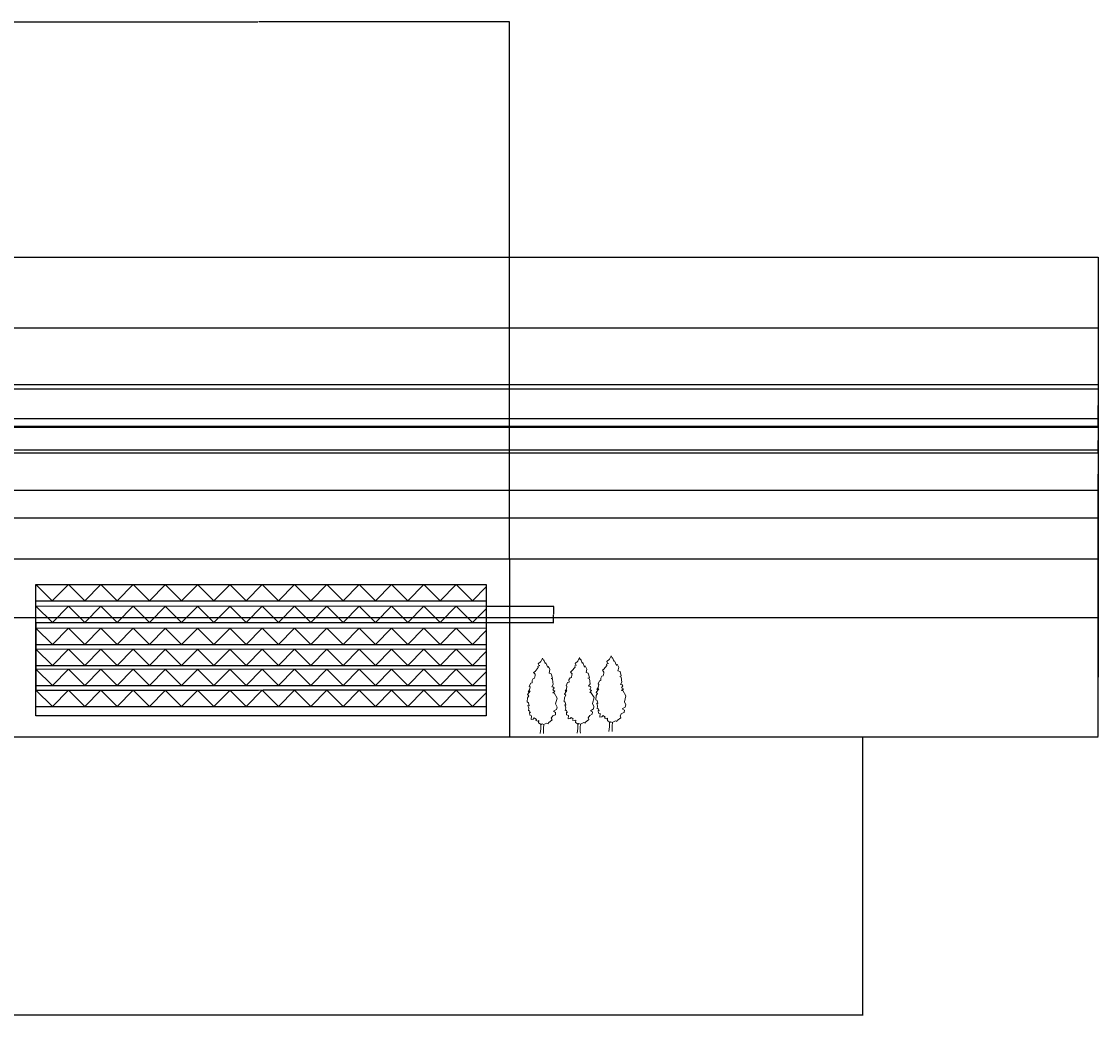
# Model space of a CAD drawing. Units: inches. Extents: x -2248 to 2617, y -128 to 922.
# Tile 7 of 7: x 1596 to 2617, y -128 to 815. Entities that reach past the tile are written whole.
import ezdxf

# ---------------------------------------------------------------- set-up
doc = ezdxf.new("R2010")
doc.units = ezdxf.units.IN
doc.header["$MEASUREMENT"] = 0
for name, color, linetype, lineweight in [('A-ANNO-DIMS', 2, 'Continuous', 18), ('A-ELEV', 7, 'Continuous', 25), ('A-ELEV-FACD', 8, 'Continuous', 13), ('L-PLNT', 3, 'Continuous', 18)]:
    doc.layers.add(name, color=color, linetype=linetype, lineweight=lineweight)
doc.styles.get("Standard").update_dxf_attribs({"font": 'arial.ttf'})
doc.dimstyles.get("Standard").update_dxf_attribs({"dimtxt": 0.18, "dimasz": 0.18, "dimexe": 0.18, "dimexo": 0.0625, "dimgap": 0.09, "dimtad": 0, "dimtih": 1, "dimtoh": 1, "dimdec": 4, "dimzin": 0, "dimdsep": 46, "dimtxsty": 'Standard', "dimcen": 0.09, "dimadec": 0, "dimazin": 0, "dimtfac": 1, "dimtdec": 4, "dimtofl": 0, "dimtmove": 0, "dimatfit": 3, "dimfxl": 1, "dimtolj": 1, "dimtzin": 0, "dimarcsym": 0})

# ---------------------------------------------------------------- blocks, each defined once
blk = doc.blocks.new('*U3')
blk.add_lwpolyline([(-2.754, 191.699), (-6.78, 182.851), (-13.682, 176.953), (-11.956, 173.266), (-9.656, 172.529), (-14.257, 170.317), (-13.682, 167.368), (-21.733, 157.783), (-25.184, 154.834), (-21.158, 150.41), (-21.733, 147.461), (-22.884, 140.825), (-26.334, 140.087), (-29.21, 134.926), (-28.635, 129.028), (-32.661, 128.291), (-36.111, 120.18), (-34.386, 118.706), (-35.536, 111.333), (-38.987, 106.171), (-34.386, 107.646), (-40.712, 98.798), (-37.261, 95.849), (-40.712, 90.688), (-41.287, 80.366), (-38.412, 78.154), (-36.686, 70.781), (-39.562, 71.518), (-37.261, 64.145), (-38.412, 57.509), (-36.111, 58.247), (-33.236, 52.348), (-35.536, 53.086), (-34.961, 46.45), (-30.36, 44.975), (-31.51, 36.128), (-26.334, 36.865), (-23.459, 39.814), (-18.283, 36.128), (-20.008, 33.178), (-14.832, 31.704), (-11.956, 33.178), (-12.531, 27.28), (-6.205, 22.856), (-3.905, 24.331), (0.121, 22.856), (8.173, 26.543), (11.624, 25.068), (12.199, 27.28), (21.4, 34.653), (19.675, 39.077), (23.701, 44.975), (30.027, 47.924), (30.602, 53.823), (25.426, 56.772), (32.903, 61.196), (34.053, 67.094), (30.602, 75.205), (34.628, 89.951), (26.576, 103.222), (23.701, 103.222), (28.302, 107.646), (23.701, 110.595), (26.576, 115.756), (25.426, 117.968), (20.825, 118.706), (24.276, 124.604), (22.551, 137.876), (19.1, 139.35), (22.551, 140.825), (19.675, 151.884), (14.499, 153.359), (16.224, 162.207), (12.199, 170.317), (10.473, 167.368), (5.872, 179.165), (4.147, 177.69), (0.696, 187.275), (-0.454, 185.8)], close=True)
for points in [[(-6.813, 23.669), (-6.813, 11.669), (-8.627, 0)], [(0.387, 23.669), (-0.576, 13.271), (-0.576, 3.686), (0, 0)]]:
    blk.add_lwpolyline(points)
blk = doc.blocks.new('FACADE-SCREEN-PANEL-2')
for p, q in [((0, 15.5), (426.7, 15.5)), ((0, 15.5), (15.6, 0)), ((15.6, 0), (30.8, 15.5)), ((30.8, 15.5), (46.4, 0)), ((46.4, 0), (61.6, 15.5)), ((61.5, 15.5), (77, 0)), ((77, 0), (92.2, 15.5)), ((92.1, 15.5), (107.7, 0)), ((107.7, 0), (122.9, 15.5)), ((122.6, 15.5), (138.1, 0)), ((138.1, 0), (153.4, 15.5)), ((153.2, 15.5), (168.8, 0)), ((168.8, 0), (184, 15.5)), ((183.8, 15.5), (199.3, 0)), ((199.3, 0), (214.5, 15.5)), ((214.4, 15.5), (230, 0)), ((230, 0), (245.2, 15.5)), ((245, 15.5), (260.5, 0)), ((260.5, 0), (275.8, 15.5)), ((275.8, 15.5), (291.3, 0)), ((291.3, 0), (306.5, 15.5)), ((306.3, 15.5), (321.9, 0)), ((321.9, 0), (337.1, 15.5)), ((337, 15.5), (352.5, 0)), ((352.5, 0), (367.7, 15.5)), ((367.6, 15.5), (383.2, 0)), ((383.2, 0), (398.4, 15.5)), ((398.3, 15.5), (413.8, 0)), ((413.8, 0), (426.7, 13.1))]:
    blk.add_line(p, q)
blk = doc.blocks.new('*D12')
at = {"layer": 'A-ANNO-DIMS', "color": 0, "lineweight": -2, "transparency": 16777216}
for p, q in [((1609.4, 244.6), (1609.4, 180.5)), ((2036.1, 244.6), (2036.1, 180.5)), ((1609.6, 180.7), (1820.5, 180.7)), ((2035.9, 180.7), (1825, 180.7))]:
    blk.add_line(p, q, dxfattribs=at)
at = {"layer": 'A-ANNO-DIMS', "color": 0, "transparency": 16777216}
for points in [[(1609.6, 180.7), (1609.6, 180.7), (1609.4, 180.7)], [(2035.9, 180.7), (2035.9, 180.7), (2036.1, 180.7)]]:
    blk.add_solid(points, dxfattribs=at)
at = {"layer": 'Defpoints', "color": 0, "transparency": 16777216}
for p in [(1609.4, 244.7), (2036.1, 244.7), (2036.1, 180.7)]:
    blk.add_point(p, dxfattribs=at)
at = {"layer": 'A-ANNO-DIMS', "color": 0, "transparency": 16777216, "insert": (1822.8, 180.7), "char_height": 0.18, "attachment_point": 5}
blk.add_mtext('\\A1;FACADE SCREEN PANEL 2 427 TYP.', dxfattribs=at)
blk = doc.blocks.new('*D13')
at = {"layer": 'A-ANNO-DIMS', "color": 0, "lineweight": -2, "transparency": 16777216}
for p, q in [((2036.2, 260.2), (2100.3, 260.2)), ((2100.1, 260), (2100.1, 252.6)), ((2100.1, 244.9), (2100.1, 252.2)), ((2036.2, 244.7), (2100.3, 244.7))]:
    blk.add_line(p, q, dxfattribs=at)
at = {"layer": 'A-ANNO-DIMS', "color": 0, "transparency": 16777216}
for points in [[(2100.1, 260), (2100.1, 260), (2100.1, 260.2)], [(2100.1, 244.9), (2100.1, 244.9), (2100.1, 244.7)]]:
    blk.add_solid(points, dxfattribs=at)
at = {"layer": 'Defpoints', "color": 0, "transparency": 16777216}
for p in [(2036.1, 260.2), (2100.1, 260.2), (2036.1, 244.7)]:
    blk.add_point(p, dxfattribs=at)
at = {"layer": 'A-ANNO-DIMS', "color": 0, "transparency": 16777216, "insert": (2100.1, 252.4), "char_height": 0.18, "attachment_point": 5}
blk.add_mtext('\\A1;15 TYP.', dxfattribs=at)
blk = doc.blocks.new('*D16')
at = {"layer": 'A-ANNO-DIMS', "color": 0, "lineweight": -2, "transparency": 16777216}
for p, q in [((45.9, 438.4), (2616.5, 438.4)), ((2616.3, 438.3), (2616.3, 287.6)), ((2616.3, 136.6), (2616.3, 287.3)), ((45.9, 136.5), (2616.5, 136.5))]:
    blk.add_line(p, q, dxfattribs=at)
at = {"layer": 'A-ANNO-DIMS', "color": 0, "transparency": 16777216}
for points in [[(2616.2, 438.3), (2616.3, 438.3), (2616.3, 438.4)], [(2616.2, 136.6), (2616.3, 136.6), (2616.3, 136.5)]]:
    blk.add_solid(points, dxfattribs=at)
at = {"layer": 'Defpoints', "color": 0, "transparency": 16777216}
for p in [(45.8, 438.4), (45.8, 136.5), (2616.3, 136.5)]:
    blk.add_point(p, dxfattribs=at)
at = {"layer": 'A-ANNO-DIMS', "color": 0, "transparency": 16777216, "insert": (2616.3, 287.4), "char_height": 0.18, "attachment_point": 5}
blk.add_mtext('\\A1;302', dxfattribs=at)
blk = doc.blocks.new('*D17')
at = {"layer": 'A-ANNO-DIMS', "color": 0, "lineweight": -2, "transparency": 16777216}
for p, q in [((625.1, 524.3), (2616.5, 524.3)), ((2616.3, 524.1), (2616.3, 330.6)), ((2616.3, 136.6), (2616.3, 330.2)), ((553.6, 136.5), (2616.5, 136.5))]:
    blk.add_line(p, q, dxfattribs=at)
at = {"layer": 'A-ANNO-DIMS', "color": 0, "transparency": 16777216}
for points in [[(2616.2, 524.1), (2616.3, 524.1), (2616.3, 524.3)], [(2616.2, 136.6), (2616.3, 136.6), (2616.3, 136.5)]]:
    blk.add_solid(points, dxfattribs=at)
at = {"layer": 'Defpoints', "color": 0, "transparency": 16777216}
for p in [(625.1, 524.3), (553.6, 136.5), (2616.3, 136.5)]:
    blk.add_point(p, dxfattribs=at)
at = {"layer": 'A-ANNO-DIMS', "color": 0, "transparency": 16777216, "insert": (2616.3, 330.4), "char_height": 0.18, "attachment_point": 5}
blk.add_mtext('\\A1;387.9', dxfattribs=at)
blk = doc.blocks.new('*D20')
at = {"layer": 'A-ANNO-DIMS', "color": 0, "lineweight": -2, "transparency": 16777216}
for p, q in [((-1595.3, 429.9), (2616.5, 429.9)), ((2616.3, 429.7), (2616.3, 417.9)), ((2616.3, 405.8), (2616.3, 417.5)), ((-1653.9, 405.6), (2616.5, 405.6))]:
    blk.add_line(p, q, dxfattribs=at)
at = {"layer": 'A-ANNO-DIMS', "color": 0, "transparency": 16777216}
for points in [[(2616.2, 429.7), (2616.3, 429.7), (2616.3, 429.9)], [(2616.2, 405.8), (2616.3, 405.8), (2616.3, 405.6)]]:
    blk.add_solid(points, dxfattribs=at)
at = {"layer": 'Defpoints', "color": 0, "transparency": 16777216}
for p in [(-1595.4, 429.9), (-1654, 405.6), (2616.3, 405.6)]:
    blk.add_point(p, dxfattribs=at)
at = {"layer": 'A-ANNO-DIMS', "color": 0, "transparency": 16777216, "insert": (2616.3, 417.7), "char_height": 0.18, "attachment_point": 5}
blk.add_mtext('\\A1;24.3', dxfattribs=at)
blk = doc.blocks.new('*D21')
at = {"layer": 'A-ANNO-DIMS', "color": 0, "lineweight": -2, "transparency": 16777216}
for p, q in [((-1125.3, 470.6), (2616.5, 470.6)), ((2616.3, 470.4), (2616.3, 451)), ((2616.3, 431.1), (2616.3, 450.6)), ((-1257.9, 430.9), (2616.5, 430.9))]:
    blk.add_line(p, q, dxfattribs=at)
at = {"layer": 'A-ANNO-DIMS', "color": 0, "transparency": 16777216}
for points in [[(2616.2, 470.4), (2616.3, 470.4), (2616.3, 470.6)], [(2616.2, 431.1), (2616.3, 431.1), (2616.3, 430.9)]]:
    blk.add_solid(points, dxfattribs=at)
at = {"layer": 'Defpoints', "color": 0, "transparency": 16777216}
for p in [(-1125.4, 470.6), (-1258, 430.9), (2616.3, 430.9)]:
    blk.add_point(p, dxfattribs=at)
at = {"layer": 'A-ANNO-DIMS', "color": 0, "transparency": 16777216, "insert": (2616.3, 450.8), "char_height": 0.18, "attachment_point": 5}
blk.add_mtext('\\A1;39.705', dxfattribs=at)
blk = doc.blocks.new('*D22')
at = {"layer": 'A-ANNO-DIMS', "color": 0, "lineweight": -2, "transparency": 16777216}
for p, q in [((-733.3, 408.4), (2616.5, 408.4)), ((2616.3, 408.2), (2616.3, 329.1)), ((2616.3, 249.6), (2616.3, 328.7)), ((-719.1, 249.4), (2616.5, 249.4))]:
    blk.add_line(p, q, dxfattribs=at)
at = {"layer": 'A-ANNO-DIMS', "color": 0, "transparency": 16777216}
for points in [[(2616.2, 408.2), (2616.3, 408.2), (2616.3, 408.4)], [(2616.2, 249.6), (2616.3, 249.6), (2616.3, 249.4)]]:
    blk.add_solid(points, dxfattribs=at)
at = {"layer": 'Defpoints', "color": 0, "transparency": 16777216}
for p in [(-733.4, 408.4), (-719.2, 249.4), (2616.3, 249.4)]:
    blk.add_point(p, dxfattribs=at)
at = {"layer": 'A-ANNO-DIMS', "color": 0, "transparency": 16777216, "insert": (2616.3, 328.9), "char_height": 0.18, "attachment_point": 5}
blk.add_mtext('\\A1;159.02', dxfattribs=at)
blk = doc.blocks.new('*D23')
at = {"layer": 'A-ANNO-DIMS', "color": 0, "lineweight": -2, "transparency": 16777216}
for p, q in [((-719.1, 249.4), (2616.5, 249.4)), ((2616.3, 249.2), (2616.3, 193.1)), ((2616.3, 136.6), (2616.3, 192.7)), ((-719.1, 136.5), (2616.5, 136.5))]:
    blk.add_line(p, q, dxfattribs=at)
at = {"layer": 'A-ANNO-DIMS', "color": 0, "transparency": 16777216}
for points in [[(2616.2, 249.2), (2616.3, 249.2), (2616.3, 249.4)], [(2616.2, 136.6), (2616.3, 136.6), (2616.3, 136.5)]]:
    blk.add_solid(points, dxfattribs=at)
at = {"layer": 'Defpoints', "color": 0, "transparency": 16777216}
for p in [(-719.2, 249.4), (-719.2, 136.5), (2616.3, 136.5)]:
    blk.add_point(p, dxfattribs=at)
at = {"layer": 'A-ANNO-DIMS', "color": 0, "transparency": 16777216, "insert": (2616.3, 192.9), "char_height": 0.18, "attachment_point": 5}
blk.add_mtext('\\A1;112.94', dxfattribs=at)
blk = doc.blocks.new('*D24')
at = {"layer": 'A-ANNO-DIMS', "color": 0, "lineweight": -2, "transparency": 16777216}
for p, q in [((-316.1, 370.3), (2616.5, 370.3)), ((2616.3, 370.1), (2616.3, 253.6)), ((2616.3, 136.6), (2616.3, 253.2)), ((-159.8, 136.5), (2616.5, 136.5))]:
    blk.add_line(p, q, dxfattribs=at)
at = {"layer": 'A-ANNO-DIMS', "color": 0, "transparency": 16777216}
for points in [[(2616.2, 370.1), (2616.3, 370.1), (2616.3, 370.3)], [(2616.2, 136.6), (2616.3, 136.6), (2616.3, 136.5)]]:
    blk.add_solid(points, dxfattribs=at)
at = {"layer": 'Defpoints', "color": 0, "transparency": 16777216}
for p in [(-316.2, 370.3), (-159.9, 136.5), (2616.3, 136.5)]:
    blk.add_point(p, dxfattribs=at)
at = {"layer": 'A-ANNO-DIMS', "color": 0, "transparency": 16777216, "insert": (2616.3, 253.4), "char_height": 0.18, "attachment_point": 5}
blk.add_mtext('\\A1;233.87', dxfattribs=at)
blk = doc.blocks.new('*D25')
at = {"layer": 'A-ANNO-DIMS', "color": 0, "lineweight": -2, "transparency": 16777216}
for p, q in [((1112.5, 344.2), (2616.5, 344.2)), ((2616.3, 344), (2616.3, 240.5)), ((2616.3, 136.6), (2616.3, 240.2)), ((1112.5, 136.5), (2616.5, 136.5))]:
    blk.add_line(p, q, dxfattribs=at)
at = {"layer": 'A-ANNO-DIMS', "color": 0, "transparency": 16777216}
for points in [[(2616.2, 344), (2616.3, 344), (2616.3, 344.2)], [(2616.2, 136.6), (2616.3, 136.6), (2616.3, 136.5)]]:
    blk.add_solid(points, dxfattribs=at)
at = {"layer": 'Defpoints', "color": 0, "transparency": 16777216}
for p in [(1112.5, 344.2), (1112.5, 136.5), (2616.3, 136.5)]:
    blk.add_point(p, dxfattribs=at)
at = {"layer": 'A-ANNO-DIMS', "color": 0, "transparency": 16777216, "insert": (2616.3, 240.3), "char_height": 0.18, "attachment_point": 5}
blk.add_mtext('\\A1;207.78', dxfattribs=at)
blk = doc.blocks.new('*D26')
at = {"layer": 'A-ANNO-DIMS', "color": 0, "lineweight": -2, "transparency": 16777216}
for p, q in [((1582.3, 466.3), (2616.5, 466.3)), ((2616.3, 466.1), (2616.3, 385.9)), ((2616.3, 305.4), (2616.3, 385.6)), ((1582.3, 305.2), (2616.5, 305.2))]:
    blk.add_line(p, q, dxfattribs=at)
at = {"layer": 'A-ANNO-DIMS', "color": 0, "transparency": 16777216}
for points in [[(2616.2, 466.1), (2616.3, 466.1), (2616.3, 466.3)], [(2616.2, 305.4), (2616.3, 305.4), (2616.3, 305.2)]]:
    blk.add_solid(points, dxfattribs=at)
at = {"layer": 'Defpoints', "color": 0, "transparency": 16777216}
for p in [(1582.2, 466.3), (1582.2, 305.2), (2616.3, 305.2)]:
    blk.add_point(p, dxfattribs=at)
at = {"layer": 'A-ANNO-DIMS', "color": 0, "transparency": 16777216, "insert": (2616.3, 385.8), "char_height": 0.18, "attachment_point": 5}
blk.add_mtext('\\A1;161.04', dxfattribs=at)
blk = doc.blocks.new('*D27')
at = {"layer": 'A-ANNO-DIMS', "color": 0, "lineweight": -2, "transparency": 16777216}
for p, q in [((2058.4, 305.2), (2616.5, 305.2)), ((2616.3, 305.1), (2616.3, 221)), ((2616.3, 136.6), (2616.3, 220.7)), ((2058.4, 136.5), (2616.5, 136.5))]:
    blk.add_line(p, q, dxfattribs=at)
at = {"layer": 'A-ANNO-DIMS', "color": 0, "transparency": 16777216}
for points in [[(2616.2, 305.1), (2616.3, 305.1), (2616.3, 305.2)], [(2616.2, 136.6), (2616.3, 136.6), (2616.3, 136.5)]]:
    blk.add_solid(points, dxfattribs=at)
at = {"layer": 'Defpoints', "color": 0, "transparency": 16777216}
for p in [(2058.4, 305.2), (2058.4, 136.5), (2616.3, 136.5)]:
    blk.add_point(p, dxfattribs=at)
at = {"layer": 'A-ANNO-DIMS', "color": 0, "transparency": 16777216, "insert": (2616.3, 220.9), "char_height": 0.18, "attachment_point": 5}
blk.add_mtext('\\A1;168.8', dxfattribs=at)
blk = doc.blocks.new('*D28')
at = {"layer": 'A-ANNO-DIMS', "color": 0, "lineweight": -2, "transparency": 16777216}
for p, q in [((1266.1, 591.3), (2616.5, 591.3)), ((2616.3, 591.1), (2616.3, 364)), ((2616.3, 136.6), (2616.3, 363.7)), ((2058.4, 136.5), (2616.5, 136.5))]:
    blk.add_line(p, q, dxfattribs=at)
at = {"layer": 'A-ANNO-DIMS', "color": 0, "transparency": 16777216}
for points in [[(2616.2, 591.1), (2616.3, 591.1), (2616.3, 591.3)], [(2616.2, 136.6), (2616.3, 136.6), (2616.3, 136.5)]]:
    blk.add_solid(points, dxfattribs=at)
at = {"layer": 'Defpoints', "color": 0, "transparency": 16777216}
for p in [(1266.1, 591.3), (2616.3, 591.3), (2058.4, 136.5)]:
    blk.add_point(p, dxfattribs=at)
at = {"layer": 'A-ANNO-DIMS', "color": 0, "transparency": 16777216, "insert": (2616.3, 363.9), "char_height": 0.18, "attachment_point": 5}
blk.add_mtext('\\A1;454.8', dxfattribs=at)
blk = doc.blocks.new('*D33')
at = {"layer": 'A-ANNO-DIMS', "color": 0, "lineweight": -2, "transparency": 16777216}
for p, q in [((2393, 136.4), (2393, -127.9)), ((-2024.3, 122), (-2024.3, -127.9)), ((-2024.1, -127.7), (184, -127.7)), ((2392.8, -127.7), (184.7, -127.7))]:
    blk.add_line(p, q, dxfattribs=at)
at = {"layer": 'A-ANNO-DIMS', "color": 0, "transparency": 16777216}
for points in [[(-2024.1, -127.6), (-2024.1, -127.7), (-2024.3, -127.7)], [(2392.8, -127.6), (2392.8, -127.7), (2393, -127.7)]]:
    blk.add_solid(points, dxfattribs=at)
at = {"layer": 'Defpoints', "color": 0, "transparency": 16777216}
for p in [(2393, 136.5), (-2024.3, 122.1), (2393, -127.7)]:
    blk.add_point(p, dxfattribs=at)
at = {"layer": 'A-ANNO-DIMS', "color": 0, "transparency": 16777216, "insert": (184.4, -127.7), "char_height": 0.18, "attachment_point": 5}
blk.add_mtext('\\A1;4417', dxfattribs=at)
blk = doc.blocks.new('*D54')
at = {"layer": 'A-ANNO-DIMS', "color": 0, "lineweight": -2, "transparency": 16777216}
for p, q in [((1582.2, 305.3), (1582.2, 814.7)), ((1582.4, 814.5), (1819.8, 814.5)), ((2058.2, 814.5), (1820.7, 814.5)), ((2058.4, 305.3), (2058.4, 814.7))]:
    blk.add_line(p, q, dxfattribs=at)
at = {"layer": 'A-ANNO-DIMS', "color": 0, "transparency": 16777216}
for points in [[(1582.4, 814.5), (1582.4, 814.5), (1582.2, 814.5)], [(2058.2, 814.5), (2058.2, 814.5), (2058.4, 814.5)]]:
    blk.add_solid(points, dxfattribs=at)
at = {"layer": 'Defpoints', "color": 0, "transparency": 16777216}
for p in [(2058.4, 814.5), (1582.2, 305.2), (2058.4, 305.2)]:
    blk.add_point(p, dxfattribs=at)
at = {"layer": 'A-ANNO-DIMS', "color": 0, "transparency": 16777216, "insert": (1820.3, 814.5), "char_height": 0.18, "attachment_point": 5}
blk.add_mtext('\\A1;476.15', dxfattribs=at)

msp = doc.modelspace()

# ---------------------------------------------------------------- linework, layer by layer
at = {"layer": 'A-ELEV'}
for p, q in [((1422.6951, 305.2491), (2058.3545, 305.2491)), ((2058.3545, 305.2491), (2058.3545, 136.4519)), ((1609.436, 280.8948), (2036.1168, 280.8948)), ((1609.436, 156.3844), (1609.436, 280.8948)), ((1609.436, 280.8948), (1625.0083, 265.4415)), ((1625.0083, 265.4415), (1640.2167, 280.8948)), ((1640.2195, 280.8948), (1655.7917, 265.4415)), ((1655.7917, 265.4415), (1671.0002, 280.8948)), ((1670.8967, 280.8948), (1686.4689, 265.4415)), ((1686.4689, 265.4415), (1701.6773, 280.8948)), ((1701.5314, 280.8948), (1717.1036, 265.4415)), ((1717.1036, 265.4415), (1732.3121, 280.8948)), ((1732.0088, 280.8948), (1747.581, 265.4415)), ((1747.581, 265.4415), (1762.7895, 280.8948)), ((1762.6712, 280.8948), (1778.2434, 265.4415)), ((1778.2434, 265.4415), (1793.4519, 280.8948)), ((1793.2024, 280.8948), (1808.7746, 265.4415)), ((1808.7746, 265.4415), (1823.9831, 280.8948)), ((1823.8798, 280.8948), (1839.452, 265.4415)), ((1839.452, 265.4415), (1854.6604, 280.8948)), ((1854.411, 280.8948), (1869.9832, 265.4415)), ((1869.9832, 265.4415), (1885.1916, 280.8948)), ((1885.186, 280.8948), (1900.7583, 265.4415)), ((1900.7583, 265.4415), (1915.9667, 280.8948)), ((1915.7173, 280.8948), (1931.2895, 265.4415)), ((1931.2895, 265.4415), (1946.4979, 280.8948)), ((1946.3893, 280.8948), (1961.9615, 265.4415)), ((1961.9615, 265.4415), (1977.17, 280.8948)), ((1977.0535, 280.8948), (1992.6258, 265.4415)), ((1992.6258, 265.4415), (2007.8342, 280.8948)), ((2007.6882, 280.8948), (2023.2605, 265.4415)), ((2023.2605, 265.4415), (2036.1168, 278.5049)), ((2036.1168, 280.8948), (2036.1168, 156.3844)), ((1609.436, 265.4415), (2036.1168, 265.4415)), ((1609.436, 244.7002), (2036.1168, 244.7002)), ((1609.436, 223.9589), (2036.1168, 223.9589)), ((1609.436, 204.0641), (2036.1168, 204.0641)), ((1609.436, 184.9313), (2036.1168, 184.9313)), ((1609.436, 165.0365), (2036.1168, 165.0365)), ((2036.1168, 156.3844), (1609.436, 156.3844)), ((1375.9892, 136.4519), (2393.0245, 136.4519))]:
    msp.add_line(p, q, dxfattribs=at)

# ---------------------------------------------------------------- block references
at = {"layer": 'A-ELEV-FACD'}
for p in [(1609.436, 244.7), (1609.436, 223.9587), (1609.436, 204.0639), (1609.436, 184.9311), (1609.436, 165.0363)]:
    msp.add_blockref('FACADE-SCREEN-PANEL-2', p, dxfattribs=at)
at = {"layer": 'L-PLNT', "xscale": 0.373818396241174, "yscale": 0.373818396241174, "zscale": 0.373818396241174}
for p in [(2090.6627, 139.4597), (2125.6176, 139.9223), (2155.791, 141.5736)]:
    msp.add_blockref('*U3', p, dxfattribs=at)

# ---------------------------------------------------------------- dimensions: what is measured, and where the dimension line sits
at = {"layer": 'A-ANNO-DIMS'}
for base, p1, p2, override, picture, middle in [((2058.3545, 814.5189), (1582.2049, 305.2491), (2058.3545, 305.2491), {"dimdec": 2, "dimlfac": 1, "dimrnd": 0, "dimzin": 0, "dimdsep": 46, "dimlunit": 2}, '*D54', (1820.2797, 814.5189)), ((2393.0245, -127.6745), (-2024.254, 122.0847), (2393.0245, 136.4519), {"dimdec": 0, "dimlfac": 1, "dimrnd": 0, "dimzin": 0, "dimdsep": 46, "dimlunit": 2}, '*D33', (184.3853, -127.6745))]:
    dim = msp.add_linear_dim(base=base, p1=p1, p2=p2, dimstyle='Standard', override=override, dxfattribs=at)
    dim.commit()
    dim.dimension.update_dxf_attribs({"geometry": picture, "text_midpoint": middle})
for base, p1, p2, override, picture, middle in [((2616.2745, 591.2689), (2058.3545, 136.4519), (1266.0706, 591.2689), {"dimdec": 1, "dimlfac": 1, "dimrnd": 0, "dimzin": 0, "dimdsep": 46, "dimlunit": 2}, '*D28', (2616.2745, 363.8604)), ((2616.2745, 136.4519), (625.0568, 524.3284), (553.5648, 136.4519), {"dimdec": 1, "dimlfac": 1, "dimrnd": 0, "dimzin": 0, "dimdsep": 46, "dimlunit": 2}, '*D17', (2616.2745, 330.3901)), ((2616.2745, 430.9238), (-1125.4072, 470.6286), (-1257.9572, 430.9238), {"dimdec": 3, "dimlfac": 1, "dimrnd": 0, "dimzin": 0, "dimdsep": 46, "dimlunit": 2}, '*D21', (2616.2745, 450.7762)), ((2616.2745, 305.2491), (1582.2049, 466.287), (1582.2049, 305.2491), {"dimdec": 2, "dimlfac": 1, "dimrnd": 0, "dimzin": 0, "dimdsep": 46, "dimlunit": 2}, '*D26', (2616.2745, 385.768)), ((2616.2745, 405.5754), (-1595.3791, 429.8743), (-1653.9599, 405.5754), {"dimdec": 1, "dimlfac": 1, "dimrnd": 0, "dimzin": 0, "dimdsep": 46, "dimlunit": 2}, '*D20', (2616.2745, 417.7249)), ((2616.2745, 136.4519), (45.827, 438.443), (45.827, 136.4519), {"dimdec": 0, "dimlfac": 1, "dimrnd": 0, "dimzin": 0, "dimdsep": 46, "dimlunit": 2}, '*D16', (2616.2745, 287.4474)), ((2616.2745, 249.389), (-733.3752, 408.4102), (-719.1936, 249.389), {"dimdec": 2, "dimlfac": 1, "dimrnd": 0, "dimzin": 0, "dimdsep": 46, "dimlunit": 2}, '*D22', (2616.2745, 328.8996)), ((2616.2745, 136.4519), (-316.2025, 370.3211), (-159.9067, 136.4519), {"dimdec": 2, "dimlfac": 1, "dimrnd": 0, "dimzin": 0, "dimdsep": 46, "dimlunit": 2}, '*D24', (2616.2745, 253.3865)), ((2616.2745, 136.4519), (1112.486, 344.2299), (1112.486, 136.4519), {"dimdec": 2, "dimlfac": 1, "dimrnd": 0, "dimzin": 0, "dimdsep": 46, "dimlunit": 2}, '*D25', (2616.2745, 240.3409)), ((2616.2745, 136.4519), (2058.3545, 305.2491), (2058.3545, 136.4519), {"dimdec": 1, "dimlfac": 1, "dimrnd": 0, "dimzin": 0, "dimdsep": 46, "dimlunit": 2}, '*D27', (2616.2745, 220.8505)), ((2616.2745, 136.4519), (-719.1936, 249.389), (-719.1936, 136.4519), {"dimdec": 2, "dimlfac": 1, "dimrnd": 0, "dimzin": 0, "dimdsep": 46, "dimlunit": 2}, '*D23', (2616.2745, 192.9204))]:
    dim = msp.add_linear_dim(base=base, p1=p1, p2=p2, angle=90, dimstyle='Standard', override=override, dxfattribs=at)
    dim.commit()
    dim.dimension.update_dxf_attribs({"geometry": picture, "text_midpoint": middle})
dim = msp.add_linear_dim(base=(2100.119, 260.1535), p1=(2036.1168, 244.7002), p2=(2036.1168, 260.1535), angle=90, text='<> TYP.', dimstyle='Standard', override={"dimdec": 0, "dimrnd": 0, "dimzin": 0, "dimlunit": 2}, dxfattribs=at)
dim.commit()
dim.dimension.update_dxf_attribs({"geometry": '*D13', "text_midpoint": (2100.119, 252.4269)})
dim = msp.add_linear_dim(base=(2036.1168, 180.6981), p1=(1609.436, 244.7002), p2=(2036.1168, 244.7002), text='FACADE SCREEN PANEL 2 <> TYP.', dimstyle='Standard', override={"dimdec": 0, "dimrnd": 0, "dimzin": 0, "dimlunit": 2}, dxfattribs=at)
dim.commit()
dim.dimension.update_dxf_attribs({"geometry": '*D12', "text_midpoint": (1822.7764, 180.6981)})

doc.saveas('drawing.dxf')
